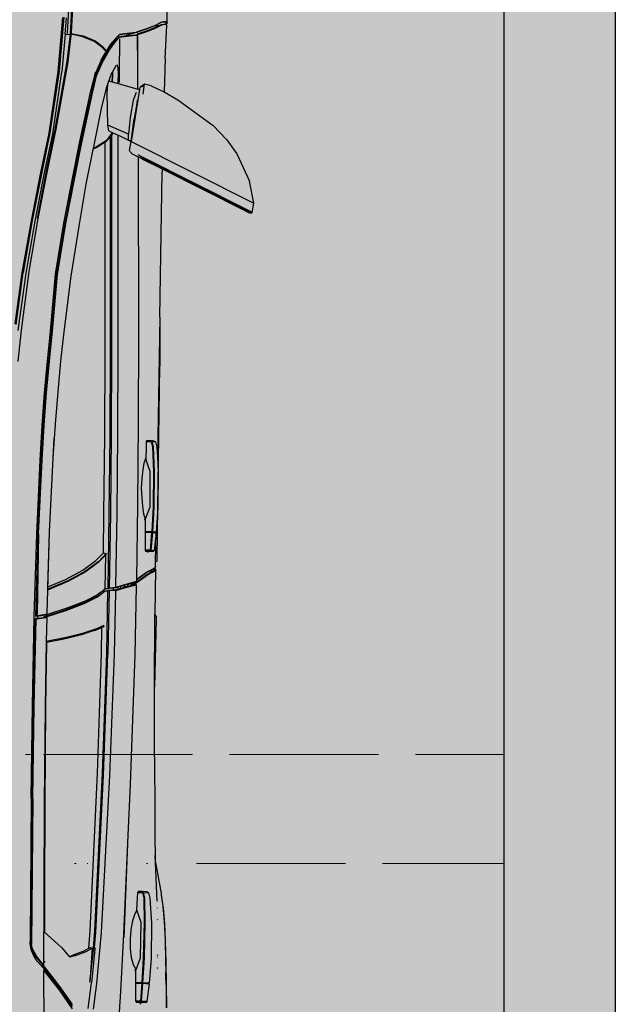
# Model space of a CAD drawing. Units: inches. Extents: x 1884 to 2398, y 474 to 1488.
# Tile 26 of 39: x 2348 to 2397, y 620 to 699. Entities that reach past the tile are written whole.
import ezdxf

# ---------------------------------------------------------------- set-up
doc = ezdxf.new("R2010")
doc.units = ezdxf.units.IN
doc.header["$MEASUREMENT"] = 0
doc.linetypes.add('ACAD_ISO02W100', pattern=[15, 12, -3])
doc.layers.get('0').update_dxf_attribs({"color": 250})
for name, color, linetype, lineweight in [('A-ANNO-DIMS', 2, 'Continuous', 18), ('A-FLOR-OVHD', 8, 'ACAD_ISO02W100', 18), ('A-WALL-PATT', 250, 'Continuous', 13), ('C-PROP', 7, 'Continuous', 30), ('C-VEHI', 8, 'Continuous', 18)]:
    doc.layers.add(name, color=color, linetype=linetype, lineweight=lineweight)
doc.layers.add('Edges', color=250, linetype='Continuous')
doc.layers.add('L-PVMT-PATT', color=9, linetype='Continuous', lineweight=13, true_color=0xc7c8ca)
doc.styles.get("Standard").update_dxf_attribs({"font": 'arial.ttf'})
doc.dimstyles.get("Standard").update_dxf_attribs({"dimtxt": 7, "dimasz": 0.18, "dimexe": 0.18, "dimexo": 0.0625, "dimgap": 0.09, "dimtad": 0, "dimtih": 1, "dimtoh": 1, "dimzin": 0, "dimdsep": 46, "dimlunit": 3, "dimtxsty": 'Standard', "dimcen": 0.09, "dimadec": 0, "dimazin": 0, "dimtfac": 1, "dimtofl": 0, "dimtmove": 0, "dimatfit": 3, "dimfxl": 1, "dimtolj": 1, "dimtzin": 0, "dimarcsym": 0})

# ---------------------------------------------------------------- blocks, each defined once
blk = doc.blocks.new('Nissan Qashqai pl')
at = {"layer": 'Edges'}
for p, q in [((8.8918, 12.7444), (9.0186, 12.9956)), ((8.9173, 12.961), (8.9731, 12.9865)), ((9.0333, 12.9845), (8.9232, 12.7662)), ((9.0386, 12.9907), (8.9254, 12.7664)), ((8.9483, 12.8082), (9.0343, 12.9785)), ((9.0186, 12.9956), (8.9731, 12.9865)), ((9.0374, 12.9925), (9.0186, 12.9956)), ((9.0356, 12.9888), (9.0333, 12.9845)), ((9.0343, 12.9785), (9.0347, 12.9794)), ((9.0347, 12.9794), (9.0362, 12.9822)), ((9.0356, 12.9888), (9.0374, 12.9925)), ((9.0362, 12.9822), (9.037, 12.9838)), ((9.0371, 12.9841), (9.037, 12.9838)), ((9.0371, 12.9841), (9.0376, 12.985)), ((9.0376, 12.985), (9.0371, 12.9847)), ((9.0386, 12.9907), (9.0374, 12.9925)), ((9.0376, 12.985), (9.0386, 12.9907)), ((8.8885, 12.9405), (8.9173, 12.961)), ((8.8591, 12.9127), (8.8879, 12.94)), ((8.8885, 12.9405), (8.8879, 12.94)), ((8.8066, 12.84), (8.8591, 12.9127)), ((8.7908, 12.812), (8.8066, 12.84)), ((8.6489, 12.8179), (8.5719, 12.8193)), ((8.646, 12.8153), (8.6489, 12.8179)), ((8.6489, 12.8179), (8.6527, 12.8156)), ((8.6547, 12.8176), (8.6537, 12.8167)), ((8.7222, 12.8144), (8.6547, 12.8176)), ((8.646, 12.8153), (8.646, 12.8153)), ((8.6472, 12.8076), (8.646, 12.8153)), ((8.647, 12.8142), (8.6498, 12.8168)), ((8.6482, 12.8067), (8.647, 12.8142)), ((8.6546, 12.7926), (8.6472, 12.8076)), ((8.655, 12.7929), (8.6482, 12.8067)), ((8.6498, 12.8168), (8.6524, 12.8153)), ((8.651, 12.814), (8.652, 12.815)), ((8.6524, 12.8064), (8.651, 12.814)), ((8.652, 12.815), (8.6524, 12.8153)), ((8.6534, 12.8073), (8.652, 12.815)), ((8.6524, 12.8153), (8.6527, 12.8156)), ((8.655, 12.801), (8.6524, 12.8064)), ((8.6527, 12.8156), (8.6537, 12.8167)), ((8.6608, 12.7921), (8.6534, 12.8073)), ((8.6537, 12.8167), (8.6537, 12.8166)), ((8.6598, 12.7913), (8.655, 12.801)), ((8.655, 12.7929), (8.655, 12.801)), ((8.7222, 12.8144), (8.7908, 12.812)), ((8.7785, 12.7855), (8.7891, 12.8089)), ((8.7891, 12.8089), (8.7908, 12.812)), ((8.928, 12.7679), (8.9483, 12.8082)), ((8.9483, 12.8082), (8.9552, 12.8081)), ((9.2517, 12.8031), (8.9552, 12.8081)), ((9.2517, 12.8031), (9.351, 12.803)), ((9.2517, 12.8031), (9.5372, 12.7983)), ((9.641, 12.7991), (9.351, 12.803)), ((9.5069, 12.7941), (9.5176, 12.7972)), ((9.5176, 12.7972), (9.5372, 12.7983)), ((9.5372, 12.7983), (9.5689, 12.7999)), ((9.5689, 12.7999), (9.641, 12.7991)), ((9.641, 12.7991), (9.6921, 12.7956)), ((9.7466, 12.7978), (9.641, 12.7991)), ((9.7511, 12.7979), (9.7466, 12.7978)), ((9.7526, 12.7946), (9.7511, 12.7979)), ((10.3679, 12.7944), (10.4275, 12.8051)), ((10.4468, 12.7976), (10.3679, 12.7944)), ((10.4275, 12.8051), (10.4304, 12.8056)), ((10.4304, 12.8056), (10.4339, 12.8061)), ((10.4339, 12.8061), (10.4573, 12.8093)), ((10.4339, 12.8061), (10.4345, 12.8062)), ((10.4345, 12.8062), (10.4613, 12.8099)), ((10.4503, 12.7976), (10.4502, 12.7976)), ((10.4573, 12.8093), (10.4889, 12.8119)), ((10.4603, 12.7976), (10.4613, 12.7978)), ((10.4613, 12.8099), (10.4926, 12.8125)), ((10.4838, 12.7977), (10.4852, 12.7982)), ((10.4889, 12.8119), (10.526, 12.8138)), ((10.4926, 12.8125), (10.5294, 12.8143)), ((10.526, 12.8138), (10.569, 12.8151)), ((10.5294, 12.8143), (10.5719, 12.8156)), ((10.5565, 12.7985), (10.5591, 12.7977)), ((10.5615, 12.7978), (10.5617, 12.7985)), ((10.569, 12.8151), (10.5919, 12.8155)), ((10.5719, 12.8156), (10.6176, 12.8164)), ((10.583, 12.7984), (10.5834, 12.798)), ((10.5836, 12.798), (10.5831, 12.7984)), ((10.5847, 12.798), (10.5841, 12.7984)), ((10.5873, 12.7981), (10.5873, 12.7981)), ((10.5919, 12.8155), (10.6151, 12.8159)), ((10.5981, 12.8157), (10.5919, 12.8155)), ((10.6174, 12.816), (10.5981, 12.8157)), ((10.6087, 12.7983), (10.6087, 12.7984)), ((10.6151, 12.8159), (10.6644, 12.8162)), ((10.6176, 12.8164), (10.6651, 12.8167)), ((8.6606, 12.7768), (8.6546, 12.7926)), ((8.6556, 12.7918), (8.655, 12.7929)), ((8.655, 12.7922), (8.655, 12.7929)), ((8.6616, 12.7758), (8.6556, 12.7918)), ((8.6657, 12.7758), (8.6598, 12.7913)), ((8.6667, 12.7584), (8.6606, 12.7768)), ((8.6667, 12.7767), (8.6608, 12.7921)), ((8.7785, 12.7855), (8.7751, 12.7719)), ((9.5037, 12.7806), (9.5045, 12.7814)), ((9.5052, 12.7918), (9.5044, 12.7856)), ((9.5044, 12.7856), (9.5045, 12.7814)), ((9.5045, 12.7814), (9.5045, 12.7759)), ((9.5052, 12.7918), (9.5069, 12.7941)), ((9.5061, 12.7878), (9.5069, 12.7941)), ((9.5168, 12.7904), (9.5061, 12.7878)), ((9.5061, 12.7856), (9.5167, 12.7883)), ((9.5063, 12.7755), (9.5061, 12.7856)), ((9.5167, 12.7883), (9.5679, 12.7899)), ((9.5679, 12.792), (9.5168, 12.7904)), ((9.5678, 12.7837), (9.5426, 12.7747)), ((9.64, 12.7831), (9.5678, 12.7837)), ((9.6401, 12.7914), (9.5679, 12.792)), ((9.5679, 12.7899), (9.64, 12.7892)), ((9.64, 12.7892), (9.6912, 12.7865)), ((9.6645, 12.7737), (9.64, 12.7831)), ((9.6913, 12.7886), (9.6401, 12.7914)), ((9.6912, 12.7811), (9.6911, 12.7796)), ((9.6911, 12.7796), (9.6911, 12.7732)), ((9.6913, 12.7886), (9.6912, 12.7865)), ((9.6912, 12.7865), (9.6912, 12.7811)), ((9.692, 12.7811), (9.6912, 12.7811)), ((9.692, 12.7943), (9.6913, 12.7886)), ((9.6921, 12.7956), (9.692, 12.7943)), ((9.6922, 12.7943), (9.692, 12.7943)), ((9.692, 12.7811), (9.6921, 12.7864)), ((9.692, 12.7796), (9.692, 12.7811)), ((9.692, 12.7733), (9.692, 12.7796)), ((9.6922, 12.7943), (9.6921, 12.7956)), ((9.7526, 12.7946), (9.6921, 12.7956)), ((9.6922, 12.7885), (9.6921, 12.7864)), ((9.6921, 12.7864), (9.7288, 12.7832)), ((9.6922, 12.7885), (9.693, 12.7955)), ((9.6922, 12.7885), (9.6922, 12.7943)), ((9.7288, 12.7854), (9.6922, 12.7885)), ((9.693, 12.7955), (9.7296, 12.7914)), ((9.7288, 12.7832), (9.7287, 12.7734)), ((9.7296, 12.7914), (9.7288, 12.7854)), ((9.7306, 12.7834), (9.7288, 12.7854)), ((9.7288, 12.7854), (9.7288, 12.7832)), ((9.7288, 12.7832), (9.7306, 12.7834)), ((9.7296, 12.7914), (9.7314, 12.7895)), ((9.7305, 12.7738), (9.7306, 12.7834)), ((9.7305, 12.7738), (9.7313, 12.7798)), ((9.7306, 12.7834), (9.7314, 12.7895)), ((9.7314, 12.7895), (9.7313, 12.7798)), ((9.733, 12.7782), (9.7313, 12.7798)), ((9.7623, 12.7945), (9.7526, 12.7946)), ((9.7623, 12.7945), (9.7643, 12.7937)), ((9.7643, 12.7937), (9.7652, 12.7927)), ((9.7643, 12.7937), (9.7648, 12.7929)), ((9.7648, 12.7929), (9.7648, 12.7929)), ((9.7648, 12.7929), (9.7664, 12.7902)), ((9.7652, 12.7927), (9.7665, 12.7907)), ((9.7665, 12.7904), (9.7664, 12.7902)), ((9.7664, 12.7902), (9.7674, 12.7885)), ((9.7667, 12.7933), (9.7665, 12.7907)), ((9.7665, 12.7907), (9.7676, 12.7889)), ((9.7677, 12.7944), (9.7667, 12.7933)), ((9.7676, 12.7931), (9.7667, 12.7933)), ((9.7673, 12.7899), (9.7676, 12.7931)), ((9.7673, 12.7897), (9.7673, 12.7899)), ((9.7673, 12.7897), (9.7676, 12.7889)), ((9.7674, 12.7885), (9.7728, 12.7781)), ((9.769, 12.7926), (9.7676, 12.7931)), ((9.7676, 12.7889), (9.7684, 12.7875)), ((9.7676, 12.7887), (9.7678, 12.7882)), ((9.7677, 12.7944), (9.7677, 12.7944)), ((9.77, 12.7936), (9.7677, 12.7944)), ((9.7677, 12.7944), (9.8598, 12.7928)), ((9.7684, 12.7875), (9.7717, 12.781)), ((9.7712, 12.7892), (9.769, 12.7926)), ((9.7734, 12.7884), (9.77, 12.7936)), ((9.7707, 12.7848), (9.7709, 12.7893)), ((9.7717, 12.781), (9.7707, 12.7848)), ((9.7709, 12.7893), (9.7712, 12.7892)), ((9.7724, 12.7874), (9.7712, 12.7892)), ((9.7717, 12.781), (9.7738, 12.7771)), ((9.7778, 12.777), (9.7724, 12.7874)), ((9.7728, 12.7781), (9.7832, 12.7637)), ((9.7788, 12.778), (9.7734, 12.7884)), ((9.7738, 12.7771), (9.7842, 12.7627)), ((9.7883, 12.7626), (9.7778, 12.777)), ((9.7894, 12.7636), (9.7788, 12.778)), ((9.8598, 12.7928), (9.8614, 12.7937)), ((9.8643, 12.7927), (9.8598, 12.7928)), ((9.8614, 12.7937), (9.8647, 12.7956)), ((10.0085, 12.7922), (9.8643, 12.7927)), ((9.8647, 12.7956), (9.869, 12.7954)), ((9.869, 12.7954), (10.0085, 12.7922)), ((10.0124, 12.7922), (10.0085, 12.7922)), ((10.1513, 12.7924), (10.0124, 12.7922)), ((10.1513, 12.7924), (10.2677, 12.793)), ((10.2677, 12.793), (10.3189, 12.7931)), ((10.3189, 12.7931), (10.3537, 12.7939)), ((10.3537, 12.7939), (10.3832, 12.7945)), ((10.3679, 12.7944), (10.3537, 12.7939)), ((10.4282, 12.7775), (10.4274, 12.7679)), ((10.4282, 12.7775), (10.4299, 12.7798)), ((10.4291, 12.77), (10.4299, 12.7798)), ((10.4299, 12.7798), (10.4406, 12.7829)), ((10.4406, 12.7829), (10.4919, 12.7858)), ((10.4919, 12.7858), (10.564, 12.7851)), ((10.564, 12.7851), (10.6151, 12.7813)), ((10.615, 12.7803), (10.6142, 12.7686)), ((10.6151, 12.7813), (10.615, 12.7803)), ((10.615, 12.7676), (10.6151, 12.7803)), ((10.6151, 12.7803), (10.615, 12.7803)), ((10.6151, 12.7803), (10.6151, 12.7813)), ((10.6151, 12.7685), (10.616, 12.7812)), ((10.616, 12.7812), (10.6526, 12.7768)), ((10.6526, 12.7768), (10.6518, 12.7657)), ((10.6526, 12.7768), (10.6543, 12.7749)), ((8.6675, 12.758), (8.6616, 12.7758)), ((8.6718, 12.7574), (8.6657, 12.7758)), ((8.6728, 12.7584), (8.6667, 12.7767)), ((8.6675, 12.758), (8.6667, 12.7584)), ((8.6679, 12.7578), (8.6675, 12.758)), ((8.6676, 12.7576), (8.6675, 12.7576)), ((8.6675, 12.7576), (8.6675, 12.7576)), ((8.6675, 12.7576), (8.6676, 12.7576)), ((8.6676, 12.7576), (8.6677, 12.7576)), ((8.6677, 12.7576), (8.6677, 12.7576)), ((8.6677, 12.7576), (8.6682, 12.7576)), ((8.6682, 12.7576), (8.6679, 12.7578)), ((8.6682, 12.7576), (8.6692, 12.7566)), ((8.6682, 12.7572), (8.6682, 12.7576)), ((8.6684, 12.7554), (8.6682, 12.7572)), ((8.6682, 12.7572), (8.6692, 12.7566)), ((8.6692, 12.7566), (8.6697, 12.7519)), ((8.6729, 12.7568), (8.6718, 12.7574)), ((8.674, 12.7578), (8.6728, 12.7584)), ((8.6733, 12.7566), (8.6729, 12.7568)), ((8.6735, 12.7544), (8.6733, 12.7566)), ((8.6742, 12.7576), (8.674, 12.7578)), ((8.6742, 12.7584), (8.6743, 12.7582)), ((8.6744, 12.755), (8.6742, 12.7576)), ((8.6744, 12.7576), (8.6742, 12.7576)), ((8.6744, 12.7578), (8.6744, 12.7576)), ((8.6773, 12.7577), (8.6744, 12.7576)), ((8.6791, 12.7578), (8.677, 12.7578)), ((8.6791, 12.7577), (8.6773, 12.7577)), ((8.7205, 12.7579), (8.6791, 12.7578)), ((8.6791, 12.7577), (8.6791, 12.7578)), ((8.6878, 12.7577), (8.6791, 12.7578)), ((8.6878, 12.7577), (8.6791, 12.7577)), ((8.6878, 12.7577), (8.6878, 12.7577)), ((8.6911, 12.7577), (8.6878, 12.7577)), ((8.7205, 12.7579), (8.6911, 12.7577)), ((8.7849, 12.7582), (8.7205, 12.7579)), ((8.7734, 12.7181), (8.7849, 12.7582)), ((8.7751, 12.7719), (8.7779, 12.7668)), ((8.7798, 12.7703), (8.7751, 12.7719)), ((8.7779, 12.7668), (8.7807, 12.763)), ((8.7798, 12.7703), (8.7807, 12.763)), ((8.7798, 12.7703), (8.7954, 12.7683)), ((8.7849, 12.7615), (8.7807, 12.763)), ((8.7849, 12.7615), (8.7858, 12.7613)), ((8.7849, 12.7582), (8.7856, 12.7608)), ((8.7858, 12.7613), (8.7856, 12.7608)), ((8.7858, 12.7613), (8.807, 12.758)), ((8.8102, 12.7568), (8.807, 12.758)), ((8.807, 12.758), (8.8918, 12.7444)), ((8.8102, 12.7568), (8.8455, 12.7506)), ((8.9171, 12.7464), (8.9233, 12.7586)), ((8.9232, 12.7662), (8.9194, 12.7588)), ((8.925, 12.762), (8.9233, 12.7586)), ((8.9233, 12.7586), (9.2886, 12.7594)), ((8.928, 12.7679), (8.925, 12.762)), ((9.2886, 12.7594), (9.4673, 12.7589)), ((9.4673, 12.7589), (9.6358, 12.7575)), ((9.5045, 12.7759), (9.5063, 12.7755)), ((9.5063, 12.7755), (9.5168, 12.7751)), ((9.5168, 12.7751), (9.5423, 12.7746)), ((9.5423, 12.7746), (9.5422, 12.7736)), ((9.5422, 12.7736), (9.5422, 12.7725)), ((9.5422, 12.7736), (9.5424, 12.7735)), ((9.5426, 12.7747), (9.5423, 12.7746)), ((9.5426, 12.7747), (9.5424, 12.7735)), ((9.5424, 12.7735), (9.5503, 12.7706)), ((9.5503, 12.7706), (9.5641, 12.7681)), ((9.5641, 12.7681), (9.5818, 12.766)), ((9.5818, 12.766), (9.6016, 12.7651)), ((9.6016, 12.7651), (9.6215, 12.766)), ((9.6215, 12.766), (9.6395, 12.7676)), ((9.6358, 12.7575), (9.7887, 12.7552)), ((9.6395, 12.7676), (9.654, 12.7697)), ((9.654, 12.7697), (9.6633, 12.7726)), ((9.6633, 12.7726), (9.6645, 12.7737)), ((9.6655, 12.7733), (9.6645, 12.7737)), ((9.6655, 12.7733), (9.6911, 12.7732)), ((9.6655, 12.7713), (9.6655, 12.7733)), ((9.6911, 12.7732), (9.692, 12.7733)), ((9.692, 12.7733), (9.7287, 12.7734)), ((9.7287, 12.7734), (9.7305, 12.7738)), ((9.7832, 12.7637), (9.7887, 12.7552)), ((9.7842, 12.7627), (9.7891, 12.7552)), ((9.7933, 12.7549), (9.7883, 12.7626)), ((9.7965, 12.7526), (9.7894, 12.7636)), ((10.4263, 12.7665), (10.4274, 12.7674)), ((10.4274, 12.7679), (10.4274, 12.7674)), ((10.4274, 12.7674), (10.4275, 12.7586)), ((10.4293, 12.7579), (10.4275, 12.7586)), ((10.4398, 12.7724), (10.4291, 12.77)), ((10.4291, 12.7677), (10.4398, 12.7701)), ((10.4293, 12.7579), (10.4291, 12.7677)), ((10.4398, 12.7573), (10.4293, 12.7579)), ((10.4909, 12.773), (10.4398, 12.7724)), ((10.4398, 12.7701), (10.4909, 12.7708)), ((10.4653, 12.7564), (10.4398, 12.7573)), ((10.4908, 12.7648), (10.4653, 12.7564)), ((10.563, 12.7633), (10.4908, 12.7648)), ((10.5631, 12.7715), (10.4909, 12.773)), ((10.4909, 12.7708), (10.563, 12.7692)), ((10.563, 12.7692), (10.6142, 12.7663)), ((10.5867, 12.7545), (10.563, 12.7633)), ((10.6142, 12.7686), (10.5631, 12.7715)), ((10.6142, 12.766), (10.6141, 12.7537)), ((10.6142, 12.7686), (10.6142, 12.7677)), ((10.6142, 12.7677), (10.615, 12.7676)), ((10.6142, 12.7677), (10.6142, 12.7663)), ((10.6142, 12.7663), (10.6142, 12.766)), ((10.6151, 12.7676), (10.615, 12.7676)), ((10.615, 12.7537), (10.6151, 12.7659)), ((10.6518, 12.7657), (10.6151, 12.7685)), ((10.6151, 12.7676), (10.6151, 12.7685)), ((10.6151, 12.7662), (10.6151, 12.7676)), ((10.6151, 12.7662), (10.6518, 12.7634)), ((10.6151, 12.7659), (10.6151, 12.7662)), ((10.6518, 12.7634), (10.6517, 12.754)), ((10.6536, 12.7639), (10.6518, 12.7657)), ((10.6518, 12.7657), (10.6518, 12.7634)), ((10.6518, 12.7634), (10.6536, 12.7639)), ((10.6543, 12.7656), (10.6535, 12.7546)), ((10.6535, 12.7546), (10.6536, 12.7639)), ((10.6536, 12.7639), (10.6537, 12.7658)), ((10.6537, 12.7658), (10.6543, 12.7749)), ((10.6537, 12.7658), (10.6543, 12.7656)), ((10.6543, 12.7749), (10.6543, 12.7656)), ((10.6578, 12.7628), (10.6543, 12.7656)), ((8.6684, 12.7554), (8.6685, 12.7549)), ((8.6684, 12.755), (8.6684, 12.7554)), ((8.6703, 12.7361), (8.6684, 12.755)), ((8.6697, 12.7519), (8.6698, 12.7516)), ((8.6714, 12.7353), (8.6697, 12.7519)), ((8.6698, 12.7516), (8.6755, 12.7343)), ((8.6754, 12.7353), (8.6735, 12.7544)), ((8.6764, 12.736), (8.6744, 12.755)), ((8.7917, 12.7547), (8.8075, 12.7486)), ((8.8075, 12.7486), (8.8429, 12.7426)), ((8.8429, 12.7426), (8.8771, 12.7388)), ((8.8918, 12.7444), (8.8455, 12.7506)), ((8.8771, 12.7388), (8.8585, 12.6969)), ((8.8895, 12.7393), (8.8771, 12.7388)), ((8.8815, 12.7228), (8.892, 12.7444)), ((8.8815, 12.7228), (8.8895, 12.7393)), ((8.8908, 12.7421), (8.8895, 12.7393)), ((8.8906, 12.7418), (8.8895, 12.7393)), ((8.8906, 12.7418), (8.8911, 12.7428)), ((8.892, 12.7444), (8.8908, 12.7421)), ((8.8911, 12.7428), (8.8919, 12.7444)), ((8.8911, 12.7428), (8.8919, 12.7444)), ((8.8919, 12.7444), (8.8911, 12.7428)), ((8.8919, 12.7444), (8.8918, 12.7444)), ((8.892, 12.7444), (8.8919, 12.7444)), ((8.8919, 12.7444), (8.8919, 12.7444)), ((8.8919, 12.7444), (8.8919, 12.7444)), ((8.9106, 12.7413), (8.892, 12.7444)), ((8.892, 12.7444), (8.892, 12.7444)), ((8.9131, 12.7421), (8.9106, 12.7413)), ((8.9171, 12.7464), (8.9131, 12.7421)), ((8.9171, 12.7464), (8.917, 12.7468)), ((9.7887, 12.7552), (9.7891, 12.7552)), ((9.7891, 12.7552), (9.79, 12.7552)), ((9.79, 12.7552), (9.7931, 12.7552)), ((9.7931, 12.7552), (9.7934, 12.7535)), ((9.7931, 12.7552), (9.7933, 12.7549)), ((9.7933, 12.7549), (9.7941, 12.7541)), ((9.7934, 12.7535), (9.7938, 12.7538)), ((9.7934, 12.7535), (9.7937, 12.7524)), ((9.7937, 12.7524), (9.7992, 12.7308)), ((9.7941, 12.7541), (9.7943, 12.7535)), ((9.7955, 12.7516), (9.7943, 12.7535)), ((9.7943, 12.7535), (9.7964, 12.7453)), ((9.7963, 12.7523), (9.7955, 12.7516)), ((9.7963, 12.7523), (9.7963, 12.7524)), ((9.7964, 12.7524), (9.7963, 12.7523)), ((9.7992, 12.7476), (9.7963, 12.7523)), ((9.7967, 12.7526), (9.7964, 12.7524)), ((9.7964, 12.7525), (9.7964, 12.7524)), ((9.7964, 12.7524), (9.7996, 12.7475)), ((9.7964, 12.7453), (9.7992, 12.7476)), ((9.7964, 12.7453), (9.7973, 12.7418)), ((9.7983, 12.7541), (9.7965, 12.7526)), ((9.7965, 12.7526), (9.7967, 12.7526)), ((9.7977, 12.7535), (9.7967, 12.7526)), ((9.7967, 12.7526), (9.7986, 12.7526)), ((9.7977, 12.7431), (9.7973, 12.7418)), ((9.7973, 12.7418), (9.7977, 12.7409)), ((9.7973, 12.7418), (9.7977, 12.7399)), ((9.7982, 12.754), (9.7977, 12.7535)), ((9.7977, 12.7444), (9.7985, 12.7451)), ((9.7985, 12.7451), (9.7977, 12.7431)), ((9.7977, 12.7431), (9.7977, 12.7444)), ((9.7977, 12.7399), (9.7977, 12.7409)), ((9.7977, 12.7409), (9.7987, 12.7388)), ((9.7977, 12.7399), (9.7978, 12.7397)), ((9.7987, 12.7388), (9.7978, 12.7397)), ((9.7978, 12.7397), (9.7987, 12.7362)), ((9.7983, 12.7541), (9.7982, 12.754)), ((9.7986, 12.7526), (9.7982, 12.754)), ((9.7986, 12.7544), (9.7983, 12.7541)), ((9.7989, 12.7461), (9.7985, 12.7451)), ((9.7993, 12.755), (9.7986, 12.7544)), ((9.7988, 12.7516), (9.7986, 12.7526)), ((9.7987, 12.7388), (9.7992, 12.7377)), ((9.7987, 12.7362), (9.7992, 12.7377)), ((9.7998, 12.7477), (9.7988, 12.7516)), ((9.7998, 12.7466), (9.7989, 12.7461)), ((9.7998, 12.7466), (9.7992, 12.7476)), ((9.7992, 12.7377), (9.8027, 12.7364)), ((9.7999, 12.7522), (9.7993, 12.755)), ((9.7993, 12.755), (9.8024, 12.7549)), ((9.7996, 12.7475), (9.7998, 12.7477)), ((9.8002, 12.7461), (9.7996, 12.7475)), ((9.8001, 12.7468), (9.7996, 12.7475)), ((9.8001, 12.7468), (9.7998, 12.7477)), ((9.8003, 12.7458), (9.7998, 12.7466)), ((9.8054, 12.7307), (9.7999, 12.7522)), ((9.8002, 12.7461), (9.8001, 12.7468)), ((9.8003, 12.7458), (9.8002, 12.7461)), ((9.8027, 12.7364), (9.8003, 12.7458)), ((9.8024, 12.7549), (9.9426, 12.7518)), ((9.9426, 12.7518), (10.2081, 12.7424)), ((10.2081, 12.7424), (10.312, 12.7377)), ((10.312, 12.7377), (10.5214, 12.7293)), ((10.312, 12.7377), (10.5147, 12.7285)), ((10.4653, 12.7561), (10.4652, 12.7545)), ((10.4653, 12.7564), (10.4653, 12.7561)), ((10.4653, 12.7564), (10.4653, 12.7564)), ((10.4653, 12.7564), (10.4653, 12.7561)), ((10.4653, 12.7561), (10.4653, 12.7561)), ((10.4653, 12.7561), (10.4732, 12.7517)), ((10.4732, 12.7517), (10.4871, 12.7474)), ((10.4871, 12.7474), (10.5048, 12.744)), ((10.5048, 12.744), (10.5246, 12.7423)), ((10.5246, 12.7423), (10.5445, 12.7425)), ((10.5445, 12.7425), (10.5625, 12.7446)), ((10.5625, 12.7446), (10.5769, 12.7484)), ((10.5769, 12.7484), (10.5863, 12.7537)), ((10.5863, 12.7537), (10.5867, 12.7545)), ((10.5885, 12.7538), (10.5867, 12.7545)), ((10.5885, 12.751), (10.5885, 12.7538)), ((10.6141, 12.7537), (10.5885, 12.7538)), ((10.6141, 12.7537), (10.615, 12.7537)), ((10.6517, 12.754), (10.615, 12.7537)), ((10.6535, 12.7546), (10.6517, 12.754)), ((8.6727, 12.7207), (8.6703, 12.7361)), ((8.6737, 12.7197), (8.6714, 12.7353)), ((8.6737, 12.7197), (8.6727, 12.7207)), ((8.6746, 12.7189), (8.6737, 12.7197)), ((8.6785, 12.7189), (8.6746, 12.7189)), ((8.6805, 12.7132), (8.6746, 12.7189)), ((8.6755, 12.7343), (8.6754, 12.7353)), ((8.6777, 12.7196), (8.6755, 12.7343)), ((8.6764, 12.7359), (8.6764, 12.736)), ((8.6788, 12.7205), (8.6764, 12.7359)), ((8.6785, 12.7189), (8.6777, 12.7196)), ((8.6815, 12.7162), (8.6785, 12.7189)), ((8.687, 12.7132), (8.6788, 12.7205)), ((8.6818, 12.7204), (8.7012, 12.7203)), ((8.7012, 12.7203), (8.7012, 12.7203)), ((8.7012, 12.7203), (8.7026, 12.7203)), ((8.7026, 12.7203), (8.7026, 12.7203)), ((8.7026, 12.7203), (8.7072, 12.7203)), ((8.7072, 12.7203), (8.7072, 12.7203)), ((8.7072, 12.7203), (8.7273, 12.7202)), ((8.7273, 12.7202), (8.7273, 12.7201)), ((8.7273, 12.7202), (8.7354, 12.7202)), ((8.7354, 12.7201), (8.7354, 12.7202)), ((8.7354, 12.7202), (8.742, 12.7202)), ((8.7415, 12.7177), (8.7361, 12.7158)), ((8.7534, 12.7185), (8.7415, 12.7177)), ((8.742, 12.7201), (8.742, 12.7202)), ((8.742, 12.7202), (8.742, 12.7201)), ((8.742, 12.7202), (8.742, 12.7202)), ((8.742, 12.7202), (8.7426, 12.7202)), ((8.7426, 12.7201), (8.7426, 12.7202)), ((8.7426, 12.7202), (8.7433, 12.7202)), ((8.7433, 12.7201), (8.7433, 12.7202)), ((8.7433, 12.7202), (8.7711, 12.7201)), ((8.7711, 12.7201), (8.7516, 12.72)), ((8.7718, 12.7181), (8.7534, 12.7185)), ((8.7698, 12.7058), (8.7734, 12.7181)), ((8.7734, 12.7181), (8.7718, 12.7181)), ((8.8734, 12.7057), (8.8793, 12.7181)), ((8.8793, 12.7181), (8.8815, 12.7228)), ((9.3194, 12.7179), (8.8793, 12.7181)), ((9.4919, 12.7173), (9.3194, 12.7179)), ((9.6538, 12.7157), (9.4919, 12.7173)), ((9.7987, 12.7362), (9.8002, 12.7301)), ((9.7992, 12.7308), (9.8044, 12.7151)), ((9.8002, 12.7301), (9.8008, 12.7285)), ((9.8008, 12.7285), (9.8014, 12.7303)), ((9.8008, 12.7285), (9.8014, 12.7265)), ((9.8014, 12.7303), (9.8031, 12.7349)), ((9.8043, 12.7303), (9.8014, 12.7303)), ((9.8014, 12.7265), (9.803, 12.723)), ((9.8014, 12.7265), (9.8026, 12.723)), ((9.803, 12.723), (9.8026, 12.723)), ((9.8026, 12.723), (9.8046, 12.7171)), ((9.8031, 12.7349), (9.8027, 12.7364)), ((9.8067, 12.7229), (9.803, 12.723)), ((9.8043, 12.7303), (9.8031, 12.7349)), ((9.8044, 12.73), (9.8043, 12.7303)), ((9.8067, 12.7229), (9.8044, 12.73)), ((9.8046, 12.7171), (9.8086, 12.7171)), ((9.8046, 12.7171), (9.8055, 12.7143)), ((9.8106, 12.715), (9.8054, 12.7307)), ((9.8086, 12.7171), (9.8067, 12.7229)), ((9.8096, 12.7142), (9.8086, 12.7171)), ((10.5147, 12.7285), (10.6318, 12.7228)), ((10.6318, 12.7228), (10.6955, 12.7184)), ((8.6805, 12.7132), (8.6884, 12.7071)), ((8.6815, 12.7162), (8.6818, 12.7154)), ((8.6817, 12.716), (8.6815, 12.7162)), ((8.6817, 12.716), (8.6818, 12.7154)), ((8.6859, 12.7122), (8.6817, 12.716)), ((8.6818, 12.7154), (8.6902, 12.7081)), ((8.6927, 12.7071), (8.6859, 12.7122)), ((8.7042, 12.7002), (8.687, 12.7132)), ((8.6917, 12.7071), (8.6884, 12.7071)), ((8.698, 12.6996), (8.6884, 12.7071)), ((8.6902, 12.7081), (8.6917, 12.7071)), ((8.6917, 12.7071), (8.7075, 12.6955)), ((8.6927, 12.7071), (8.6923, 12.7071)), ((8.7032, 12.6992), (8.6927, 12.7071)), ((8.7071, 12.6942), (8.698, 12.6996)), ((8.7302, 12.684), (8.7032, 12.6992)), ((8.7312, 12.6851), (8.7042, 12.7002)), ((8.7361, 12.7158), (8.7373, 12.7128)), ((8.7373, 12.7128), (8.7492, 12.7059)), ((8.7492, 12.7059), (8.7572, 12.7062)), ((8.7492, 12.7059), (8.7524, 12.704)), ((8.7524, 12.704), (8.7828, 12.6934)), ((8.7572, 12.7062), (8.7698, 12.7058)), ((8.7698, 12.7057), (8.7583, 12.706)), ((8.7678, 12.6988), (8.7698, 12.7057)), ((8.7748, 12.6967), (8.7678, 12.6988)), ((8.7698, 12.7057), (8.7698, 12.7058)), ((8.7916, 12.6954), (8.7748, 12.6967)), ((8.8585, 12.6969), (8.8259, 12.6959)), ((8.87, 12.6987), (8.8585, 12.6969)), ((8.87, 12.6987), (8.8734, 12.7057)), ((8.8734, 12.7057), (8.8768, 12.7057)), ((8.8751, 12.7054), (8.8768, 12.7057)), ((8.8893, 12.6956), (8.8751, 12.7054)), ((8.8768, 12.7057), (8.879, 12.704)), ((8.879, 12.704), (9.3198, 12.7039)), ((8.879, 12.704), (8.881, 12.7023)), ((9.3225, 12.7021), (8.881, 12.7023)), ((8.881, 12.7023), (8.8893, 12.6956)), ((9.3198, 12.7039), (9.4922, 12.7033)), ((9.4936, 12.7013), (9.3225, 12.7021)), ((9.4922, 12.7033), (9.654, 12.7018)), ((9.6552, 12.6997), (9.4936, 12.7013)), ((9.802, 12.7133), (9.6538, 12.7157)), ((9.654, 12.7018), (9.8061, 12.6994)), ((9.8078, 12.6971), (9.6552, 12.6997)), ((9.8051, 12.7132), (9.802, 12.7133)), ((9.8044, 12.7151), (9.8051, 12.7132)), ((9.8061, 12.6994), (9.8051, 12.7132)), ((9.8055, 12.7143), (9.8058, 12.7073)), ((9.8058, 12.7073), (9.8098, 12.7073)), ((9.8058, 12.7073), (9.8061, 12.6994)), ((9.8061, 12.6994), (9.8078, 12.6971)), ((9.8078, 12.6971), (9.8078, 12.6913)), ((9.8098, 12.7073), (9.8096, 12.7142)), ((9.8101, 12.6993), (9.8098, 12.7073)), ((9.8101, 12.6993), (9.8112, 12.7131)), ((9.8119, 12.697), (9.8101, 12.6993)), ((9.8101, 12.6993), (9.9411, 12.6966)), ((9.8112, 12.7131), (9.8106, 12.715)), ((9.8143, 12.713), (9.8112, 12.7131)), ((9.9393, 12.6944), (9.8119, 12.697)), ((9.8119, 12.6912), (9.8119, 12.697)), ((9.9414, 12.71), (9.8143, 12.713)), ((10.1894, 12.6879), (9.9411, 12.6966)), ((10.19, 12.7008), (9.9414, 12.71)), ((10.5113, 12.6839), (10.19, 12.7008)), ((8.6864, 12.6706), (8.697, 12.685)), ((8.6875, 12.6698), (8.6979, 12.6839)), ((8.6924, 12.676), (8.6883, 12.6704)), ((8.6987, 12.6845), (8.6924, 12.676)), ((8.6924, 12.676), (8.6924, 12.6762)), ((8.697, 12.685), (8.7055, 12.6927)), ((8.6979, 12.6839), (8.7062, 12.6915)), ((8.7062, 12.6915), (8.6987, 12.6845)), ((8.7055, 12.6927), (8.7071, 12.6942)), ((8.7062, 12.6915), (8.7067, 12.6919)), ((8.7067, 12.6919), (8.7083, 12.6934)), ((8.7071, 12.6942), (8.7083, 12.6934)), ((8.7075, 12.6955), (8.7346, 12.6806)), ((8.7083, 12.6934), (8.7083, 12.6934)), ((8.7083, 12.6934), (8.7083, 12.6934)), ((8.7102, 12.6923), (8.7083, 12.6934)), ((8.7083, 12.6934), (8.7083, 12.6934)), ((8.7108, 12.6919), (8.7102, 12.6923)), ((8.7102, 12.6923), (8.7102, 12.6923)), ((8.7257, 12.6833), (8.7108, 12.6919)), ((8.7248, 12.6836), (8.7108, 12.6919)), ((8.7257, 12.6833), (8.7248, 12.6836)), ((8.7257, 12.6832), (8.7257, 12.6833)), ((8.7257, 12.6832), (8.7508, 12.672)), ((8.7529, 12.6741), (8.7302, 12.684)), ((8.7574, 12.6737), (8.7312, 12.6851)), ((8.7346, 12.6806), (8.7491, 12.6738)), ((8.7346, 12.6806), (8.7577, 12.6709)), ((8.7828, 12.6934), (8.8245, 12.6828)), ((8.8259, 12.6959), (8.7916, 12.6954)), ((8.8245, 12.6828), (8.9063, 12.6663)), ((8.8893, 12.6956), (8.9021, 12.6745)), ((8.8913, 12.6936), (8.8893, 12.6956)), ((8.8927, 12.6913), (8.8913, 12.6936)), ((9.3224, 12.6911), (8.8927, 12.6913)), ((8.9041, 12.6725), (8.8927, 12.6913)), ((9.3225, 12.6911), (9.3224, 12.6911)), ((9.4936, 12.6904), (9.3225, 12.6911)), ((9.6552, 12.6888), (9.4936, 12.6904)), ((9.7337, 12.6875), (9.6552, 12.6888)), ((9.7337, 12.6875), (9.7357, 12.6935)), ((9.7499, 12.6721), (9.7337, 12.6875)), ((9.7357, 12.6935), (9.7378, 12.6924)), ((9.7357, 12.6935), (9.7519, 12.678)), ((9.7378, 12.6924), (9.754, 12.677)), ((9.8078, 12.6913), (9.7378, 12.6924)), ((9.7519, 12.678), (9.7713, 12.6512)), ((9.754, 12.677), (9.7733, 12.6502)), ((9.8078, 12.6913), (9.8119, 12.6862)), ((9.8241, 12.6756), (9.8119, 12.6912)), ((9.8119, 12.6862), (9.8119, 12.6912)), ((9.8147, 12.6826), (9.8119, 12.6862)), ((9.8147, 12.6826), (9.8147, 12.6826)), ((9.8147, 12.6826), (9.8201, 12.6756)), ((9.8241, 12.6706), (9.8147, 12.6826)), ((9.8891, 12.6741), (9.8818, 12.6891)), ((9.8867, 12.6842), (9.8838, 12.6901)), ((9.9393, 12.684), (9.8867, 12.6842)), ((9.8911, 12.675), (9.8867, 12.6842)), ((10.1849, 12.6857), (9.9393, 12.6944)), ((10.1849, 12.6754), (9.9393, 12.684)), ((10.5079, 12.6703), (10.1849, 12.6857)), ((10.5109, 12.6721), (10.1894, 12.6879)), ((10.6152, 12.674), (10.5113, 12.6839)), ((8.6759, 12.6459), (8.6864, 12.6706)), ((8.6772, 12.6454), (8.6875, 12.6698)), ((8.6883, 12.6704), (8.6777, 12.6457)), ((8.7508, 12.672), (8.7491, 12.6738)), ((8.7491, 12.6738), (8.7576, 12.6699)), ((8.7532, 12.6708), (8.7508, 12.672)), ((8.7529, 12.6741), (8.7577, 12.6709)), ((8.757, 12.6724), (8.7529, 12.6741)), ((8.7575, 12.6698), (8.7532, 12.6708)), ((8.7587, 12.672), (8.757, 12.6724)), ((8.7931, 12.6653), (8.7574, 12.6737)), ((8.7576, 12.6699), (8.7575, 12.6698)), ((8.7881, 12.6621), (8.7575, 12.6698)), ((8.7582, 12.6707), (8.7576, 12.6699)), ((8.7577, 12.6709), (8.7582, 12.6707)), ((8.759, 12.6717), (8.7582, 12.6707)), ((8.7587, 12.672), (8.759, 12.6717)), ((8.7591, 12.6719), (8.7587, 12.672)), ((8.7591, 12.6719), (8.759, 12.6717)), ((8.7925, 12.664), (8.7591, 12.6719)), ((8.8918, 12.6392), (8.7881, 12.6621)), ((8.8941, 12.6418), (8.7925, 12.664)), ((8.8942, 12.6432), (8.7931, 12.6653)), ((8.8083, 12.6591), (8.8954, 12.6403)), ((8.9021, 12.6745), (8.9063, 12.6663)), ((8.9075, 12.6661), (8.9041, 12.6725)), ((8.9063, 12.6663), (8.9075, 12.6661)), ((8.9075, 12.6661), (8.9087, 12.6658)), ((8.9087, 12.6658), (8.9797, 12.6518)), ((9.7692, 12.6453), (9.7499, 12.6721)), ((9.8201, 12.6756), (9.8338, 12.6486)), ((9.8378, 12.6485), (9.8241, 12.6756)), ((9.8378, 12.6435), (9.8241, 12.6706)), ((9.8978, 12.6472), (9.8891, 12.6741)), ((9.8911, 12.6749), (9.8911, 12.675)), ((9.8931, 12.6691), (9.8911, 12.6749)), ((9.8911, 12.6749), (9.8998, 12.6481)), ((9.8931, 12.669), (9.8931, 12.6691)), ((9.8931, 12.669), (9.9018, 12.6421)), ((10.5079, 12.6607), (10.1849, 12.6754)), ((10.543, 12.6671), (10.5079, 12.6703)), ((10.543, 12.6576), (10.5079, 12.6607)), ((10.5417, 12.6693), (10.5109, 12.6721)), ((10.5417, 12.6693), (10.5427, 12.6702)), ((10.5417, 12.6693), (10.543, 12.6671)), ((10.5436, 12.6687), (10.5427, 12.6702)), ((10.5427, 12.6702), (10.5458, 12.67)), ((10.544, 12.6678), (10.543, 12.6671)), ((10.543, 12.6646), (10.543, 12.6671)), ((10.543, 12.6646), (10.543, 12.6576)), ((10.5439, 12.6646), (10.543, 12.6646)), ((10.5502, 12.6526), (10.543, 12.6646)), ((10.5502, 12.6456), (10.543, 12.6576)), ((10.544, 12.6678), (10.5436, 12.6687)), ((10.5439, 12.6646), (10.613, 12.6601)), ((10.547, 12.6674), (10.544, 12.6678)), ((10.5458, 12.67), (10.6144, 12.6629)), ((10.613, 12.6601), (10.547, 12.6674)), ((10.6664, 12.6566), (10.6144, 12.6629)), ((10.6678, 12.6672), (10.6152, 12.674)), ((8.6716, 12.6242), (8.6759, 12.6459)), ((8.6772, 12.6454), (8.6721, 12.6201)), ((8.6777, 12.6457), (8.6727, 12.6213)), ((8.9679, 12.6241), (8.8918, 12.6392)), ((9.0601, 12.6092), (8.8941, 12.6418)), ((8.9696, 12.6285), (8.8942, 12.6432)), ((8.8961, 12.6401), (8.9704, 12.6257)), ((8.9797, 12.6518), (9.0656, 12.6372)), ((9.0656, 12.6372), (9.1676, 12.6212)), ((9.7885, 12.6099), (9.7692, 12.6453)), ((9.7713, 12.6512), (9.7905, 12.6158)), ((9.7733, 12.6502), (9.7925, 12.6148)), ((9.8338, 12.6486), (9.8475, 12.613)), ((9.8516, 12.6129), (9.8378, 12.6485)), ((9.8516, 12.6079), (9.8378, 12.6435)), ((9.9066, 12.6119), (9.8978, 12.6472)), ((9.9086, 12.6129), (9.8998, 12.6481)), ((9.9018, 12.6421), (9.9106, 12.6068)), ((10.5584, 12.6306), (10.5502, 12.6526)), ((10.5502, 12.6456), (10.5584, 12.6236)), ((8.6197, 12.6241), (8.6683, 12.6215)), ((8.6721, 12.6201), (8.6204, 12.6229)), ((8.622, 12.6161), (8.6699, 12.6132)), ((8.6683, 12.6215), (8.671, 12.6214)), ((8.671, 12.6214), (8.6716, 12.6242)), ((8.671, 12.6214), (8.6721, 12.6201)), ((8.6727, 12.6213), (8.6721, 12.6201)), ((8.6733, 12.6129), (8.6721, 12.6201)), ((8.7287, 12.6134), (8.6721, 12.6201)), ((8.6727, 12.6213), (8.6753, 12.621)), ((8.6753, 12.621), (8.7292, 12.6146)), ((9.0591, 12.6065), (8.9679, 12.6241)), ((9.06, 12.6106), (8.9696, 12.6285)), ((8.9704, 12.6257), (8.9708, 12.6256)), ((8.9708, 12.6256), (9.0143, 12.6169)), ((9.1676, 12.6212), (9.2814, 12.6065)), ((9.7905, 12.6158), (9.8087, 12.574)), ((10.5419, 12.6018), (10.56, 12.6176)), ((10.5584, 12.6306), (10.5617, 12.619)), ((10.56, 12.6176), (10.5584, 12.6236)), ((10.56, 12.6176), (10.5617, 12.619)), ((10.6583, 12.6245), (10.6215, 12.5986)), ((10.6627, 12.6241), (10.6261, 12.5984)), ((10.6306, 12.5982), (10.6671, 12.6238)), ((8.6375, 12.6066), (8.7481, 12.5968)), ((8.6386, 12.6037), (8.7491, 12.594)), ((8.6721, 12.6093), (8.6387, 12.6123)), ((8.6699, 12.6132), (8.6721, 12.613)), ((8.6721, 12.6127), (8.6721, 12.613)), ((8.6721, 12.613), (8.6733, 12.6129)), ((8.6721, 12.6093), (8.6733, 12.6129)), ((8.6721, 12.6093), (8.7496, 12.6025)), ((8.8666, 12.5888), (8.7287, 12.6134)), ((8.7292, 12.6146), (8.8666, 12.5901)), ((8.7481, 12.5968), (8.8745, 12.5782)), ((8.8761, 12.5839), (8.7496, 12.6025)), ((9.1639, 12.5895), (9.0591, 12.6065)), ((9.1644, 12.5938), (9.06, 12.6106)), ((9.1645, 12.5924), (9.0601, 12.6092)), ((9.2814, 12.6065), (9.3416, 12.5999)), ((9.3416, 12.5999), (9.4048, 12.5941)), ((9.8039, 12.5741), (9.7885, 12.6099)), ((9.7925, 12.6148), (9.8107, 12.573)), ((9.8475, 12.613), (9.8611, 12.5708)), ((9.8652, 12.5704), (9.8516, 12.6129)), ((9.8652, 12.5654), (9.8516, 12.6079)), ((9.9149, 12.5705), (9.9066, 12.6119)), ((9.9169, 12.5714), (9.9086, 12.6129)), ((9.9106, 12.6068), (9.9177, 12.5714)), ((10.51, 12.5666), (10.5419, 12.6018)), ((10.6215, 12.5986), (10.5796, 12.5655)), ((10.5892, 12.5659), (10.6306, 12.5982)), ((10.6261, 12.5984), (10.593, 12.5726)), ((8.7491, 12.594), (8.8754, 12.5755)), ((8.8666, 12.5901), (8.9521, 12.5726)), ((8.9522, 12.5713), (8.8666, 12.5888)), ((8.8745, 12.5782), (8.9583, 12.5609)), ((8.8754, 12.5755), (8.9591, 12.5583)), ((8.9598, 12.5666), (8.8761, 12.5839)), ((9.1393, 12.5951), (9.1647, 12.591)), ((9.2801, 12.5794), (9.1639, 12.5895)), ((9.2803, 12.5836), (9.1644, 12.5938)), ((9.2804, 12.5821), (9.1645, 12.5924)), ((9.1647, 12.591), (9.1668, 12.5908)), ((9.1668, 12.5908), (9.2019, 12.5877)), ((9.3418, 12.5729), (9.2801, 12.5794)), ((9.3418, 12.5771), (9.2803, 12.5836)), ((9.3419, 12.5756), (9.2804, 12.5821)), ((9.4062, 12.5713), (9.3418, 12.5771)), ((9.4063, 12.5699), (9.3419, 12.5756)), ((9.4048, 12.5941), (9.471, 12.5888)), ((9.471, 12.5888), (9.4997, 12.5869)), ((9.5404, 12.5844), (9.4997, 12.5869)), ((9.4997, 12.5869), (9.5403, 12.5842)), ((9.5403, 12.5842), (9.6913, 12.5767)), ((9.6912, 12.5774), (9.5404, 12.5844)), ((9.8039, 12.5741), (9.6912, 12.5774)), ((9.6913, 12.5767), (9.8099, 12.573)), ((8.9521, 12.5726), (9.0495, 12.5536)), ((9.0497, 12.5523), (8.9522, 12.5713)), ((8.9583, 12.5609), (9.0538, 12.5419)), ((8.9591, 12.5583), (9.0546, 12.5394)), ((9.0552, 12.5477), (8.9598, 12.5666)), ((9.4064, 12.5671), (9.3418, 12.5729)), ((9.4735, 12.5663), (9.4062, 12.5713)), ((9.4736, 12.5648), (9.4063, 12.5699)), ((9.4739, 12.5621), (9.4064, 12.5671)), ((9.5437, 12.5619), (9.4735, 12.5663)), ((9.5438, 12.5605), (9.4736, 12.5648)), ((9.5443, 12.5579), (9.4739, 12.5621)), ((9.6953, 12.5549), (9.5437, 12.5619)), ((9.6954, 12.5535), (9.5438, 12.5605)), ((9.696, 12.551), (9.5443, 12.5579)), ((9.8087, 12.574), (9.8039, 12.5741)), ((9.8099, 12.573), (9.8087, 12.574)), ((9.8099, 12.573), (9.8107, 12.573)), ((9.8107, 12.573), (9.8573, 12.5716)), ((9.8573, 12.5716), (9.8603, 12.5715)), ((9.8603, 12.5715), (9.8605, 12.5696)), ((9.8611, 12.5708), (9.8603, 12.5715)), ((9.8605, 12.5696), (9.8626, 12.5564)), ((9.8612, 12.5707), (9.8611, 12.5708)), ((9.8612, 12.5707), (9.8615, 12.5688)), ((9.8615, 12.5688), (9.8635, 12.5556)), ((9.8626, 12.5564), (9.8627, 12.5532)), ((9.8635, 12.5556), (9.8637, 12.5532)), ((9.8652, 12.5706), (9.8664, 12.5714)), ((9.8652, 12.5706), (9.8665, 12.5695)), ((9.8652, 12.5704), (9.8652, 12.5706)), ((9.8652, 12.5704), (9.8652, 12.5704)), ((9.8652, 12.5704), (9.8652, 12.5654)), ((9.8655, 12.5687), (9.8652, 12.5704)), ((9.8675, 12.5555), (9.8655, 12.5687)), ((9.8665, 12.5695), (9.8664, 12.5714)), ((9.8664, 12.5714), (9.9149, 12.5705)), ((9.8686, 12.5562), (9.8665, 12.5695)), ((9.8677, 12.5531), (9.8675, 12.5555)), ((9.8689, 12.5515), (9.8686, 12.5562)), ((9.9149, 12.5705), (10.0505, 12.5681)), ((9.9177, 12.5714), (9.9169, 12.5714)), ((10.0501, 12.5695), (9.9177, 12.5714)), ((10.2453, 12.568), (10.0501, 12.5695)), ((10.0505, 12.5681), (10.2453, 12.5664)), ((10.4292, 12.5674), (10.2453, 12.568)), ((10.2453, 12.5664), (10.4289, 12.5658)), ((10.4289, 12.5658), (10.5092, 12.5658)), ((10.5099, 12.5674), (10.4292, 12.5674)), ((10.5099, 12.5674), (10.5092, 12.5658)), ((10.5092, 12.5658), (10.5094, 12.5658)), ((10.5094, 12.5658), (10.51, 12.5666)), ((10.5783, 12.5659), (10.5094, 12.5658)), ((10.51, 12.5666), (10.5099, 12.5674)), ((10.5764, 12.5642), (10.5598, 12.5507)), ((10.5776, 12.5633), (10.5612, 12.5498)), ((10.5834, 12.5641), (10.57, 12.5517)), ((10.57, 12.5517), (10.5821, 12.5633)), ((10.5709, 12.5675), (10.5705, 12.5671)), ((10.5719, 12.5682), (10.5709, 12.5675)), ((10.5783, 12.5659), (10.5764, 12.5642)), ((10.5776, 12.5633), (10.5783, 12.5659)), ((10.5796, 12.5655), (10.5776, 12.5633)), ((10.5796, 12.5655), (10.5783, 12.5659)), ((10.5796, 12.562), (10.5796, 12.5655)), ((10.5838, 12.5653), (10.5821, 12.5633)), ((10.584, 12.5647), (10.5834, 12.5641)), ((10.584, 12.5655), (10.5838, 12.5653)), ((10.593, 12.5726), (10.584, 12.5655)), ((10.584, 12.5655), (10.5841, 12.5655)), ((10.584, 12.5654), (10.584, 12.5655)), ((10.5847, 12.5655), (10.584, 12.5647)), ((10.584, 12.5647), (10.584, 12.5654)), ((10.5851, 12.5659), (10.5841, 12.5655)), ((10.5841, 12.5655), (10.5847, 12.5655)), ((10.5851, 12.5659), (10.5847, 12.5655)), ((10.5851, 12.5659), (10.5892, 12.5659)), ((10.6988, 12.5662), (10.5892, 12.5659)), ((9.0495, 12.5536), (9.1584, 12.5351)), ((9.0538, 12.5419), (9.1605, 12.5233)), ((9.0546, 12.5394), (9.1612, 12.5208)), ((9.1617, 12.5292), (9.0552, 12.5477)), ((9.1584, 12.5351), (9.2783, 12.5191)), ((9.6953, 12.5549), (9.8598, 12.5517)), ((9.6953, 12.5549), (9.863, 12.5497)), ((9.6954, 12.5535), (9.8641, 12.5483)), ((9.8644, 12.5459), (9.696, 12.551)), ((9.8629, 12.5516), (9.8598, 12.5517)), ((9.8637, 12.5532), (9.8627, 12.5532)), ((9.8627, 12.5532), (9.8629, 12.5516)), ((9.8629, 12.5516), (9.863, 12.5497)), ((9.8641, 12.5483), (9.863, 12.5497)), ((9.8643, 12.5532), (9.8637, 12.5532)), ((9.8637, 12.5532), (9.8638, 12.5508)), ((9.8638, 12.5508), (9.8641, 12.5483)), ((9.8677, 12.5531), (9.8643, 12.5532)), ((10.0472, 12.5423), (9.8644, 12.5459)), ((9.8678, 12.5507), (9.8677, 12.5531)), ((9.8681, 12.5482), (9.8678, 12.5507)), ((9.8681, 12.5482), (9.869, 12.5496)), ((10.0476, 12.5445), (9.8681, 12.5482)), ((9.869, 12.5496), (9.8689, 12.5515)), ((10.0477, 12.5459), (9.869, 12.5496)), ((10.2357, 12.5398), (10.0472, 12.5423)), ((10.2367, 12.5419), (10.0476, 12.5445)), ((10.2369, 12.5433), (10.0477, 12.5459)), ((10.2357, 12.5398), (10.53, 12.5373)), ((10.2367, 12.5419), (10.5351, 12.5392)), ((10.2369, 12.5433), (10.5348, 12.5406)), ((10.4153, 12.5384), (10.4176, 12.5384)), ((10.4176, 12.5384), (10.4181, 12.5384)), ((10.4181, 12.5384), (10.4552, 12.538)), ((10.4181, 12.5384), (10.4181, 12.5384)), ((10.4778, 12.5378), (10.53, 12.5373)), ((10.5301, 12.5373), (10.53, 12.5373)), ((10.5335, 12.5378), (10.5301, 12.5373)), ((10.5419, 12.5391), (10.5335, 12.5378)), ((10.5422, 12.542), (10.5348, 12.5406)), ((10.5418, 12.5405), (10.5351, 12.5392)), ((10.5424, 12.5406), (10.5418, 12.5405)), ((10.5419, 12.5391), (10.5463, 12.541)), ((10.5479, 12.54), (10.5419, 12.5391)), ((10.5522, 12.5465), (10.5422, 12.542)), ((10.5495, 12.5438), (10.5424, 12.5406)), ((10.5463, 12.541), (10.5551, 12.5457)), ((10.5589, 12.5451), (10.5479, 12.54)), ((10.5546, 12.546), (10.5495, 12.5438)), ((10.5598, 12.5507), (10.5522, 12.5465)), ((10.5583, 12.5481), (10.5546, 12.546)), ((10.5551, 12.5457), (10.5583, 12.5481)), ((10.5612, 12.5498), (10.5583, 12.5481)), ((10.57, 12.5517), (10.5589, 12.5451)), ((9.2669, 12.5088), (9.1605, 12.5233)), ((9.1612, 12.5208), (9.2656, 12.5065)), ((9.2789, 12.5131), (9.1617, 12.5292)), ((9.2783, 12.5191), (9.3422, 12.5126))]:
    blk.add_line(p, q, dxfattribs=at)
blk = doc.blocks.new('car')
blk.add_blockref('Nissan Qashqai pl', (-9.7433, -11.9151))
blk = doc.blocks.new('carr')
blk.add_blockref('car', (0.5124, -0.007))
blk = doc.blocks.new('*D49')
at = {"layer": 'A-ANNO-DIMS', "color": 0, "lineweight": -2, "transparency": 16777216}
for p, q in [((2318.409, 987.716), (2318.409, 484.005)), ((2340.409, 987.716), (2340.409, 484.005)), ((2318.589, 484.185), (2340.229, 484.185)), ((2340.409, 484.185), (2340.589, 484.185))]:
    blk.add_line(p, q, dxfattribs=at)
at = {"layer": 'A-ANNO-DIMS', "color": 0, "lineweight": 100, "transparency": 16777216}
for points in [[(2318.589, 484.215), (2318.589, 484.155), (2318.409, 484.185)], [(2340.229, 484.215), (2340.229, 484.155), (2340.409, 484.185)]]:
    blk.add_solid(points, dxfattribs=at)
at = {"layer": 'Defpoints', "color": 0, "lineweight": 100, "transparency": 16777216}
for p in [(2318.409, 987.778), (2340.409, 987.778), (2340.409, 484.185)]:
    blk.add_point(p, dxfattribs=at)
at = {"layer": 'A-ANNO-DIMS', "color": 0, "transparency": 16777216, "insert": (2352.373, 484.185), "char_height": 7, "attachment_point": 5}
blk.add_mtext('\\A1;1\'-10"', dxfattribs=at)

msp = doc.modelspace()

# ---------------------------------------------------------------- hatches: boundary and pattern name
at = {"layer": 'A-WALL-PATT'}
h = msp.add_hatch(color=256, dxfattribs=at)
h.dxf.hatch_style = 1
h.paths.add_polyline_path([(2351.529, 837.963), (2342.529, 837.963), (2342.529, 813.478), (2351.529, 813.478)])
h.paths.add_polyline_path([(2351.529, 782.175), (2342.529, 782.175), (2342.529, 778.966), (2238.447, 778.966), (2238.447, 769.966), (2351.529, 769.966)])
h.paths.add_polyline_path([(2351.529, 914.773), (2342.529, 914.773), (2342.529, 901.966), (2222.529, 901.966), (2222.529, 908.236), (2213.529, 908.236), (2213.529, 901.966), (2198.529, 901.966), (2198.529, 892.966), (2198.529, 815.857), (2203.029, 815.857), (2203.029, 892.966), (2342.529, 892.966), (2342.529, 869.555), (2346.047, 869.555), (2351.529, 869.555), (2351.529, 880.385)])
h.paths.add_polyline_path([(2208.948, 778.966), (2203.029, 778.966), (2203.029, 782.647), (2198.529, 782.647), (2198.529, 779.109), (2193.526, 779.109), (2193.526, 769.966), (2198.529, 769.966), (2208.948, 769.966)])
h.paths.add_polyline_path([(2126.529, 815.801), (2117.529, 815.801), (2117.529, 676.183), (2126.529, 676.183), (2126.529, 769.966), (2132.515, 769.966), (2132.515, 778.664), (2126.529, 778.664)])
h.paths.add_polyline_path([(2135.996, 901.385), (2009.529, 901.385), (2009.529, 929.544), (2000.529, 929.544), (2000.529, 892.385), (2117.529, 892.385), (2117.529, 880.382), (2126.529, 880.382), (2126.529, 892.385), (2135.996, 892.385)])
h.paths.add_polyline_path([(2198.529, 901.385), (2185.2, 901.385), (2185.2, 892.385), (2198.529, 892.385), (2198.529, 892.966)])
h.paths.add_polyline_path([(1961.529, 892.385), (1965.143, 892.385), (1965.143, 901.385), (1952.529, 901.385), (1952.529, 604.13), (1961.529, 604.13), (1961.529, 631.385), (1988.002, 631.385), (1988.002, 640.385), (1961.529, 640.385)])
h.paths.add_polyline_path([(1955.529, 604.13), (1952.529, 604.13), (1952.529, 530.885), (2126.529, 530.885), (2126.529, 533.885), (1955.529, 533.885)])
h.paths.add_polyline_path([(2396.529, 604.13), (2393.529, 604.13), (2393.529, 533.885), (2126.529, 533.885), (2126.529, 530.885), (2396.529, 530.885)])
h.paths.add_polyline_path([(2396.529, 779.322), (2387.529, 779.322), (2387.529, 604.13), (2396.529, 604.13)])
at = {"layer": 'L-PVMT-PATT'}
h = msp.add_hatch(color=256, dxfattribs=at)
h.dxf.hatch_style = 1
h.paths.add_polyline_path([(2387.529, 769.966), (2351.529, 769.966), (2238.447, 769.966), (2238.447, 762.15), (2238.447, 754.445), (2126.529, 754.445), (2126.529, 676.183), (2134.868, 676.183), (2142.673, 676.183), (2142.673, 646.578), (2134.868, 646.578), (2126.529, 646.578), (2126.529, 640.17), (2387.529, 640.17)])
h.paths.add_polyline_path([(2387.529, 631.385), (2303.086, 631.385), (2303.086, 615.671), (2387.529, 615.671)])
h.paths.add_polyline_path([(2387.529, 640.17), (2126.529, 640.17), (2126.529, 631.385), (2387.529, 631.385)])
h.paths.add_polyline_path([(2393.529, 604.13), (2387.529, 604.13), (2387.529, 615.671), (2303.086, 615.671), (2303.086, 607.943), (2249.649, 607.943), (2126.529, 607.943), (2126.529, 533.885), (2393.529, 533.885)])
h.paths.add_polyline_path([(2257.825, 611.008), (2257.83, 611.337), (2257.915, 616.493), (2258.021, 621.805), (2258.146, 627.274), (2258.252, 631.385), (2126.529, 631.385), (2126.529, 611.008)])
h.paths.add_polyline_path([(2258.892, 611.285), (2258.888, 611.008), (2300.247, 611.008), (2300.247, 631.385), (2259.314, 631.385), (2259.206, 627.173), (2259.081, 621.72), (2258.976, 616.424)])

# ---------------------------------------------------------------- linework, layer by layer
at = {"layer": 'A-FLOR-OVHD'}
for p, q in [((2348.966, 640.17), (2349.366, 640.17)), ((2350.428, 640.17), (2387.529, 640.17)), ((2349.1, 631.385), (2349.104, 631.385)), ((2352.915, 631.385), (2353.057, 631.385)), ((2353.935, 631.385), (2353.987, 631.385)), ((2358.737, 631.385), (2358.828, 631.385)), ((2362.765, 631.385), (2387.529, 631.385))]:
    msp.add_line(p, q, dxfattribs=at)
at = {"layer": 'C-PROP'}
for p, q in [((2396.529, 1406.885), (2396.529, 530.885)), ((2387.529, 779.322), (2387.529, 604.13))]:
    msp.add_line(p, q, dxfattribs=at)

# ---------------------------------------------------------------- block references
at = {"layer": 'C-VEHI', "xscale": 39.37007874015748, "yscale": 39.37007874015748, "zscale": 39.37007874015748, "rotation": 270}
msp.add_blockref('carr', (2325.111, 676.232), dxfattribs=at)

# ---------------------------------------------------------------- dimensions: what is measured, and where the dimension line sits
at = {"layer": 'A-ANNO-DIMS'}
dim = msp.add_linear_dim(base=(2340.409, 484.185), p1=(2318.409, 987.778), p2=(2340.409, 987.778), dimstyle='Standard', override={"dimdec": 1, "dimlfac": 1, "dimrnd": 0, "dimzin": 1, "dimdsep": 46, "dimlunit": 4, "dimfrac": 2}, dxfattribs=at)
dim.commit()
dim.dimension.update_dxf_attribs({"geometry": '*D49', "text_midpoint": (2352.373, 484.185)})

doc.saveas('drawing.dxf')
